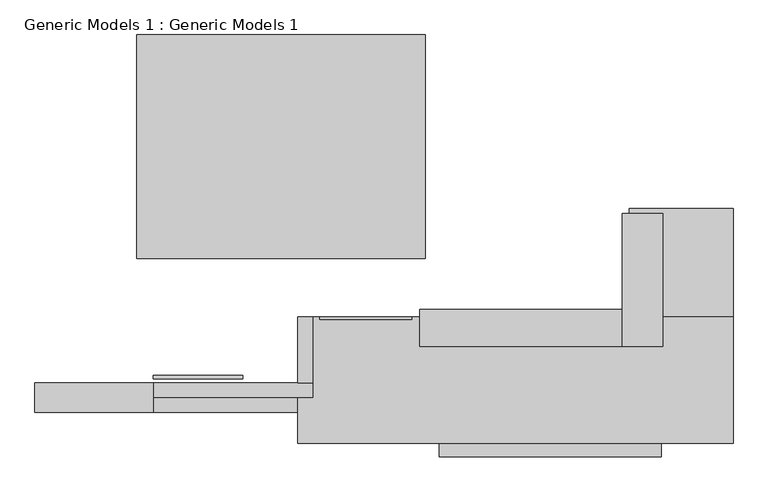
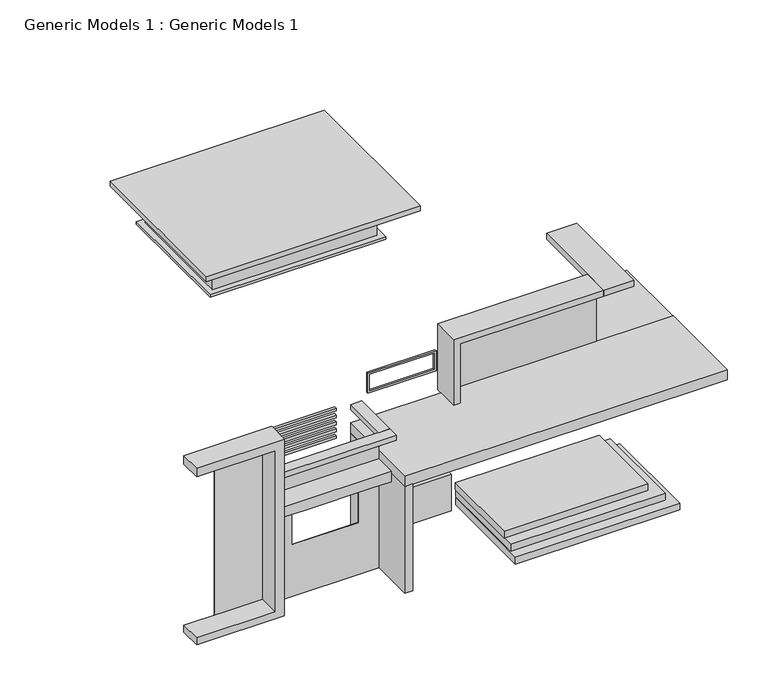
"""IFC4 building model written with IfcOpenShell, lengths in millimetres: proxy geometry, Generic Models 1 : Generic Models 1."""

from ifc_helpers import new_model, si_unit, frame, origin, origin_with_axes, place, context, project, spatial, polyline, outline, extrude, faceted_brep, source, transform, mapped, element, save


def generic_models_1_generic_models_1_dd7d6be2(model_context):
    return source(origin(), model_context, "Body", "SolidModel", [
        extrude(outline(polyline([(66.6635932, 7891.6874556), (66.6635932, 3282.6957931), (-5869.6928023, 3282.6957931), (-5869.6928023, 7891.6874556), (66.6635932, 7891.6874556)])), frame((0.0, 0.0, 8001.0), z_axis=(0.0, 0.0, 1.0), x_axis=(1.0, 0.0, 0.0)), (0.0, 0.0, 1.0), 152.4),
        faceted_brep([(-695.3364068, 7282.0874556, 8001.0), (-5260.0928023, 7282.0874556, 8001.0), (-5260.0928023, 4044.6957931, 8001.0), (-695.3364068, 4044.6957931, 8001.0), (-695.3364068, 7282.0874556, 7086.6), (-695.3364068, 4044.6957931, 7086.6), (-5260.0928023, 4044.6957931, 7086.6), (-5260.0928023, 7282.0874556, 7086.6), (-796.9364068, 4146.2957931, 7086.6), (-796.9364068, 7180.4874556, 7086.6), (-5158.4928023, 7180.4874556, 7086.6), (-5158.4928023, 4146.2957931, 7086.6), (-796.9364068, 7180.4874556, 7998.7179688), (-796.9364068, 4146.2957931, 7998.7179688), (-5158.4928023, 4146.2957931, 7998.7179688), (-5158.4928023, 7180.4874556, 7998.7179688)], [[[0, 1, 2, 3]], [[4, 5, 6, 7], [8, 9, 10, 11]], [[1, 0, 4, 7]], [[2, 1, 7, 6]], [[3, 2, 6, 5]], [[0, 3, 5, 4]], [[12, 13, 14, 15]], [[13, 12, 9, 8]], [[14, 13, 8, 11]], [[15, 14, 11, 10]], [[12, 15, 10, 9]]]),
        extrude(outline(polyline([(-542.9364068, 7434.4874556), (-542.9364068, 3892.2957931), (-5412.4928023, 3892.2957931), (-5412.4928023, 7434.4874556), (-542.9364068, 7434.4874556)])), frame((0.0, 0.0, 7010.4), z_axis=(0.0, 0.0, 1.0), x_axis=(1.0, 0.0, 0.0)), (0.0, 0.0, 1.0), 76.2),
        extrude(outline(polyline([(3810.0, -2554.9928023), (3810.0, -5526.7928023), (0.0, -5526.7928023), (0.0, -2554.9928023), (3810.0, -2554.9928023)]), holes=[polyline([(2743.2, -3126.4928023), (1524.0, -3126.4928023), (1524.0, -4955.2928023), (2743.2, -4955.2928023), (2743.2, -3126.4928023)])]), frame((0.0, 727.7137619, 0.0), z_axis=(0.0, 1.0, 0.0), x_axis=(0.0, 0.0, 1.0)), (0.0, 0.0, 1.0), 2.2820312),
        extrude(outline(polyline([(-5780.7928023, 727.7137619), (-7126.9928023, 727.7137619), (-7126.9928023, 729.9957931), (-5780.7928023, 729.9957931), (-5780.7928023, 727.7137619)])), frame((0.0, 0.0, 203.2), z_axis=(0.0, 0.0, 1.0), x_axis=(1.0, 0.0, 0.0)), (0.0, 0.0, 1.0), 4663.6970985),
        extrude(outline(polyline([(4264.9071977, 2080.2637619), (105.0780197, 2080.2637619), (105.0780197, 2082.5457931), (4264.9071977, 2082.5457931), (4264.9071977, 2080.2637619)])), frame((0.0, 0.0, 3419.199671), z_axis=(0.0, 0.0, 1.0), x_axis=(1.0, 0.0, 0.0)), (0.0, 0.0, 1.0), 1610.000329),
        extrude(outline(polyline([(378.7071977, -209.5497473), (378.7071977, 2133.3457931), (4372.1187458, 2133.3457931), (4372.1187458, -209.5497473), (378.7071977, -209.5497473)])), frame((0.0, 0.0, 406.4), z_axis=(0.0, 0.0, 1.0), x_axis=(1.0, 0.0, 0.0)), (0.0, 0.0, 1.0), 203.2),
        extrude(outline(polyline([(384.3187458, -514.3497473), (384.3187458, 2127.2502527), (4676.9187458, 2127.2502527), (4676.9187458, -514.3497473), (384.3187458, -514.3497473)])), frame((0.0, 0.0, 203.2), z_axis=(0.0, 0.0, 1.0), x_axis=(1.0, 0.0, 0.0)), (0.0, 0.0, 1.0), 203.2),
        extrude(outline(polyline([(4917.640629, -794.9309249), (357.7023948, -794.9309249), (357.7023948, 2082.5457931), (4917.640629, 2082.5457931), (4917.640629, -794.9309249)])), origin_with_axes(), (0.0, 0.0, 1.0), 203.2),
        extrude(outline(polyline([(150.1071977, 1930.1457931), (-2326.3928023, 1930.1457931), (-2326.3928023, 2082.5457931), (150.1071977, 2082.5457931), (150.1071977, 1930.1457931)])), origin_with_axes(), (0.0, 0.0, 1.0), 1066.8),
        extrude(outline(polyline([(4171.95, -2108.1683725), (4171.95, -216.2084578), (4756.15, -216.2084578), (4756.15, -2108.1683725), (4171.95, -2108.1683725)]), holes=[polyline([(4705.35, -267.0084578), (4222.75, -267.0084578), (4222.75, -2057.3683725), (4705.35, -2057.3683725), (4705.35, -267.0084578)])]), frame((0.0, 2031.7457931, 0.0), z_axis=(0.0, 1.0, 0.0), x_axis=(0.0, 0.0, 1.0)), (0.0, 0.0, 1.0), 50.8),
        extrude(outline(polyline([(-3687.4832719, 882.3957931), (-3687.4832719, 806.1957931), (-5526.7928023, 806.1957931), (-5526.7928023, 882.3957931), (-3687.4832719, 882.3957931)])), frame((0.0, 0.0, 4953.0), z_axis=(0.0, 0.0, 1.0), x_axis=(1.0, 0.0, 0.0)), (0.0, 0.0, 1.0), 76.2),
        extrude(outline(polyline([(-3687.4832719, 882.3957931), (-3687.4832719, 806.1957931), (-5526.7928023, 806.1957931), (-5526.7928023, 882.3957931), (-3687.4832719, 882.3957931)])), frame((0.0, 0.0, 4749.8), z_axis=(0.0, 0.0, 1.0), x_axis=(1.0, 0.0, 0.0)), (0.0, 0.0, 1.0), 76.2),
        extrude(outline(polyline([(-3687.4832719, 882.3957931), (-3687.4832719, 806.1957931), (-5526.7928023, 806.1957931), (-5526.7928023, 882.3957931), (-3687.4832719, 882.3957931)])), frame((0.0, 0.0, 4546.6), z_axis=(0.0, 0.0, 1.0), x_axis=(1.0, 0.0, 0.0)), (0.0, 0.0, 1.0), 76.2),
        extrude(outline(polyline([(-3687.4832719, 882.3957931), (-3687.4832719, 806.1957931), (-5526.7928023, 806.1957931), (-5526.7928023, 882.3957931), (-3687.4832719, 882.3957931)])), frame((0.0, 0.0, 4343.4), z_axis=(0.0, 0.0, 1.0), x_axis=(1.0, 0.0, 0.0)), (0.0, 0.0, 1.0), 76.2),
        extrude(outline(polyline([(-3687.4832719, 882.3957931), (-3687.4832719, 806.1957931), (-5526.7928023, 806.1957931), (-5526.7928023, 882.3957931), (-3687.4832719, 882.3957931)])), frame((0.0, 0.0, 4140.2), z_axis=(0.0, 0.0, 1.0), x_axis=(1.0, 0.0, 0.0)), (0.0, 0.0, 1.0), 76.2),
        extrude(outline(polyline([(6397.4461913, 4311.3957931), (6397.4461913, 2082.5457931), (4264.9071977, 2082.5457931), (4264.9071977, 4311.3957931), (6397.4461913, 4311.3957931)])), frame((0.0, 0.0, 3127.6644013), z_axis=(0.0, 0.0, 1.0), x_axis=(1.0, 0.0, 0.0)), (0.0, 0.0, 1.0), 291.5352697),
        extrude(outline(polyline([(4950.7071977, 1472.9457931), (4112.5071977, 1472.9457931), (4112.5071977, 4216.1457931), (4950.7071977, 4216.1457931), (4950.7071977, 1472.9457931)])), frame((0.0, 0.0, 5181.6), z_axis=(0.0, 0.0, 1.0), x_axis=(1.0, 0.0, 0.0)), (0.0, 0.0, 1.0), 177.8),
        extrude(outline(polyline([(3420.9971763, 131.0571977), (5181.6, 131.0571977), (5181.6, 4112.5071977), (5359.4, 4112.5071977), (5359.4, -46.7428023), (3420.9971763, -46.7428023), (3420.9971763, 131.0571977)])), frame((0.0, 1472.9457931, 0.0), z_axis=(0.0, 1.0, 0.0), x_axis=(0.0, 0.0, 1.0)), (0.0, 0.0, 1.0), 762.0),
        extrude(outline(polyline([(-2326.3928023, -514.6042069), (-2554.9928023, -514.6042069), (-2554.9928023, 2082.5457931), (-2326.3928023, 2082.5457931), (-2326.3928023, -514.6042069)])), origin_with_axes(), (0.0, 0.0, 1.0), 3127.6644013),
        extrude(outline(polyline([(6397.4461913, -514.6042069), (-2554.9928023, -514.6042069), (-2554.9928023, 2082.5457931), (6397.4461913, 2082.5457931), (6397.4461913, -514.6042069)])), frame((0.0, 0.0, 3127.6644013), z_axis=(0.0, 0.0, 1.0), x_axis=(1.0, 0.0, 0.0)), (0.0, 0.0, 1.0), 304.8),
        extrude(outline(polyline([(-2250.1928023, 2082.5457931), (-2250.1928023, 729.9957931), (-2554.9928023, 729.9957931), (-2554.9928023, 2082.5457931), (-2250.1928023, 2082.5457931)])), frame((0.0, 0.0, 3810.0), z_axis=(0.0, 0.0, 1.0), x_axis=(1.0, 0.0, 0.0)), (0.0, 0.0, 1.0), 152.4),
        extrude(outline(polyline([(-2250.1928023, 425.1957931), (-5526.7928023, 425.1957931), (-5526.7928023, 729.9957931), (-2250.1928023, 729.9957931), (-2250.1928023, 425.1957931)])), frame((0.0, 0.0, 3810.0), z_axis=(0.0, 0.0, 1.0), x_axis=(1.0, 0.0, 0.0)), (0.0, 0.0, 1.0), 152.4),
        extrude(outline(polyline([(0.0, -5526.7928023), (5181.6, -5526.7928023), (5181.6, -7965.1928023), (4927.6, -7965.1928023), (4927.6, -5780.7928023), (203.2, -5780.7928023), (203.2, -7965.1928023), (0.0, -7965.1928023), (0.0, -5526.7928023)])), frame((0.0, 120.3957931, 0.0), z_axis=(0.0, 1.0, 0.0), x_axis=(0.0, 0.0, 1.0)), (0.0, 0.0, 1.0), 609.6),
        extrude(outline(polyline([(2895.6, -2554.9928023), (3200.4, -2554.9928023), (3200.4, -5526.7928023), (2895.6, -5526.7928023), (2895.6, -4955.2928023), (2895.6, -3126.4928023), (2895.6, -2554.9928023)])), frame((0.0, 120.3957931, 0.0), z_axis=(0.0, 1.0, 0.0), x_axis=(0.0, 0.0, 1.0)), (0.0, 0.0, 1.0), 609.6),
    ])


if __name__ == "__main__":
    model = new_model("IFC4")
    model_context = context("Model", 3, world=origin())
    ifc_project = project(units=[si_unit("LENGTHUNIT", "METRE", prefix="MILLI")], contexts=[model_context])
    site = spatial("IfcSite", under=ifc_project)
    building = spatial("IfcBuilding", under=site)
    placement = place(None, origin())
    generic_models_1_generic_models_1_shape = generic_models_1_generic_models_1_dd7d6be2(model_context)
    element("IfcBuildingElementProxy", 1, Name="Generic Models 1 : Generic Models 1", ObjectType="Generic Models 1 : Generic Models 1", at=placement, inside=building, context=model_context, shape_type="MappedRepresentation", body=[
        mapped(generic_models_1_generic_models_1_shape, transform((0.0, 0.0, 0.0), x_axis=(1.0, 0.0, 0.0), y_axis=(0.0, 1.0, 0.0), z_axis=(0.0, 0.0, 1.0))),
    ])
    save(model, "model.ifc")

# Revit data of these elements
# Element 1 (IfcBuildingElementProxy, "Generic Models 1 : Generic Models 1")
#   Materials on its faces: "Gypsum Wall Board", "window wall", "wood up", "Roofing, EPDM Membrane", "black tile", "wood material", "black"
# Materials
#   "Gypsum Wall Board": class "Generic", colour RGB 127 127 127, transparency 0, Description = "Gypsum Wall Board", Cost = 0
#   "window wall": class "Generic", colour RGB 120 120 120, transparency 0, Cost = 0
#   "wood up": class "Generic", colour RGB 120 120 120, transparency 0, Cost = 0
#   "Roofing, EPDM Membrane": class "Generic", colour RGB 127 127 127, transparency 0, Description = "EPDM roof membrane", Cost = 0
#   "black tile": class "Generic", colour RGB 120 120 120, transparency 0, Cost = 0
#   "wood material": class "Generic", colour RGB 120 120 120, transparency 0, Cost = 0
#   "black": class "Generic", colour RGB 120 120 120, transparency 0, Cost = 0
